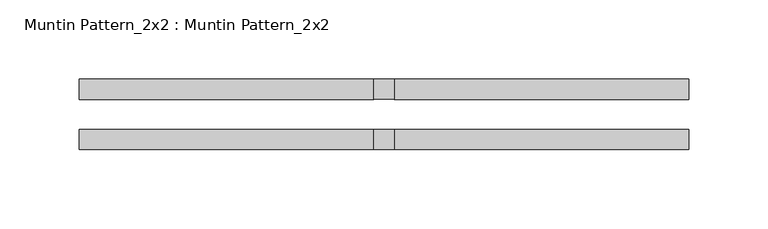
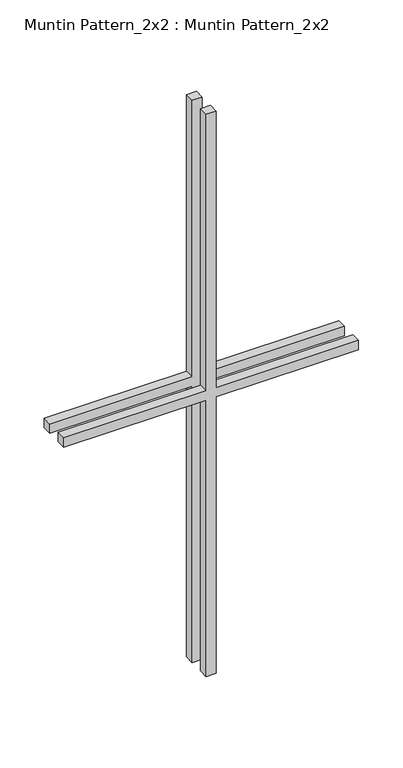
"""IFC4 building model written with IfcOpenShell, lengths in millimetres: proxy geometry, Muntin Pattern_2x2 : Muntin Pattern_2x2."""

from ifc_helpers import new_model, si_unit, frame, origin, place, context, project, spatial, polyline, outline, extrude, source, transform, mapped, element, save


def muntin_pattern_2x2_muntin_pattern_2x2_972acb6d(model_context):
    return source(origin(), model_context, "Body", "SweptSolid", [
        extrude(outline(polyline([(393.7, -6.35), (393.7, -192.0875), (381.0, -192.0875), (381.0, -6.35), (0.0, -6.35), (0.0, 6.35), (381.0, 6.35), (381.0, 192.0875), (393.7, 192.0875), (393.7, 6.35), (774.7, 6.35), (774.7, -6.35), (393.7, -6.35)])), frame((0.0, -22.225, 0.0), z_axis=(0.0, 1.0, 0.0), x_axis=(0.0, 0.0, 1.0)), (0.0, 0.0, 1.0), 12.7),
        extrude(outline(polyline([(393.7, -6.35), (393.7, -192.0875), (381.0, -192.0875), (381.0, -6.35), (0.0, -6.35), (0.0, 6.35), (381.0, 6.35), (381.0, 192.0875), (393.7, 192.0875), (393.7, 6.35), (774.7, 6.35), (774.7, -6.35), (393.7, -6.35)])), frame((0.0, 9.525, 0.0), z_axis=(0.0, 1.0, 0.0), x_axis=(0.0, 0.0, 1.0)), (0.0, 0.0, 1.0), 12.7),
    ])


if __name__ == "__main__":
    model = new_model("IFC4")
    model_context = context("Model", 3, world=origin())
    ifc_project = project(units=[si_unit("LENGTHUNIT", "METRE", prefix="MILLI")], contexts=[model_context])
    site = spatial("IfcSite", under=ifc_project)
    building = spatial("IfcBuilding", under=site)
    placement = place(None, origin())
    muntin_pattern_2x2_muntin_pattern_2x2_shape = muntin_pattern_2x2_muntin_pattern_2x2_972acb6d(model_context)
    element("IfcBuildingElementProxy", 1, Name="Muntin Pattern_2x2 : Muntin Pattern_2x2", ObjectType="Muntin Pattern_2x2 : Muntin Pattern_2x2", at=placement, inside=building, context=model_context, shape_type="MappedRepresentation", body=[
        mapped(muntin_pattern_2x2_muntin_pattern_2x2_shape, transform((0.0, 0.0, 0.0), x_axis=(1.0, 0.0, 0.0), y_axis=(0.0, 1.0, 0.0), z_axis=(0.0, 0.0, 1.0))),
    ])
    save(model, "model.ifc")

# Revit data of these elements
# Type "Muntin Pattern_2x2 : Muntin Pattern_2x2"
#   Width [instance default] = 4' - 0"
#   Thickness = 0' - 0 1/2"
#   Height [instance default] = 4' - 0"
#   Distance = 0' - 0 3/4"
#   Interior Material [instance default] = none
#   Exterior Material [instance default] = none
#   Default Elevation = 0
# Element 1 (IfcBuildingElementProxy, "Muntin Pattern_2x2 : Muntin Pattern_2x2")
#   Width = 1' - 3 1/8"
#   Height = 2' - 6 1/2"
#   Interior Material = Wood - Stained
#   Exterior Material = Clad - White
#   Materials on its faces: "Clad - White", "Wood - Stained"
# Materials
#   "Clad - White": class "Wood", colour RGB 242 242 238, transparency 0, Cost = 0
#   "Wood - Stained": class "Wood", colour RGB 224 178 126, transparency 0, Cost = 0
